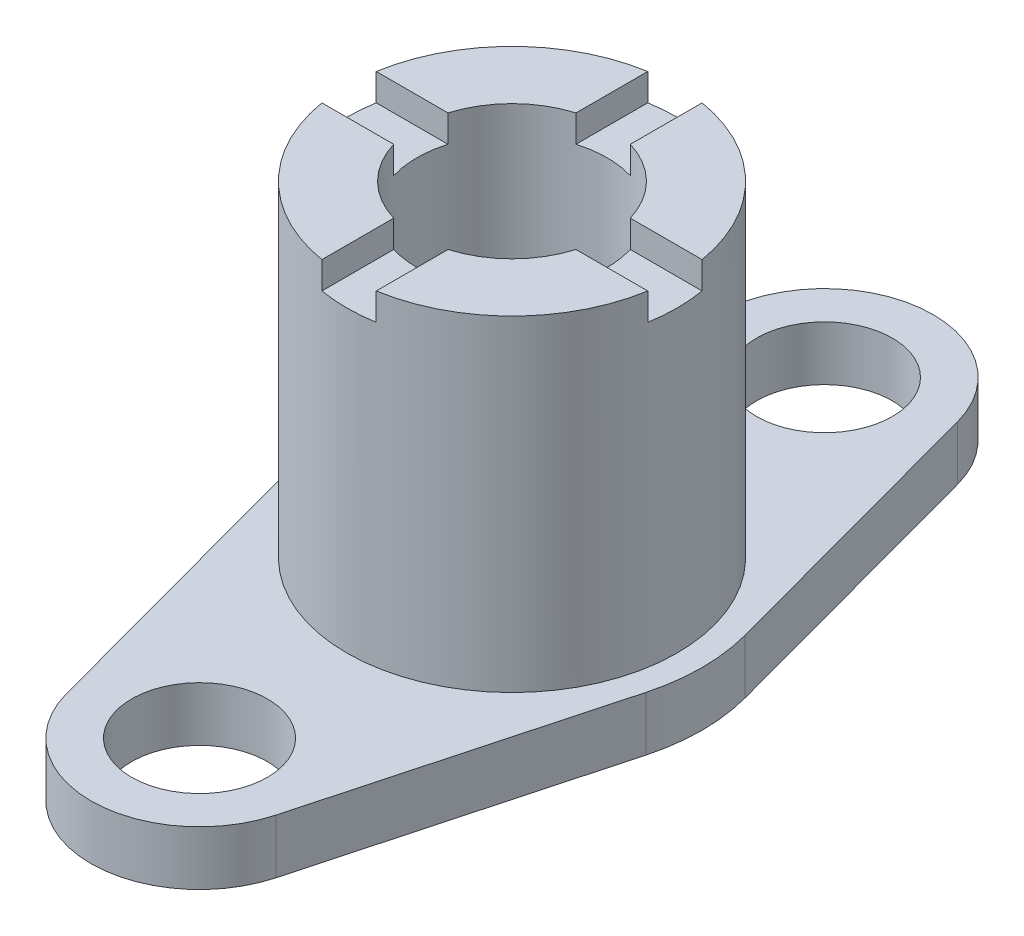
ISO-10303-21;
HEADER;
FILE_DESCRIPTION(('STEP AP214'),'2;1');
FILE_NAME('part.step','',(''),(''),'','','');
FILE_SCHEMA(('AUTOMOTIVE_DESIGN { 1 0 10303 214 1 1 1 1 }'));
ENDSEC;
DATA;
#1=APPLICATION_CONTEXT('core data for automotive mechanical design processes');
#2=APPLICATION_PROTOCOL_DEFINITION('international standard','automotive_design',2000,#1);
#3=PRODUCT_CONTEXT('',#1,'mechanical');
#4=PRODUCT('Part','Part','',(#3));
#5=PRODUCT_RELATED_PRODUCT_CATEGORY('part','',(#4));
#6=PRODUCT_DEFINITION_FORMATION('','',#4);
#7=PRODUCT_DEFINITION_CONTEXT('part definition',#1,'design');
#8=PRODUCT_DEFINITION('design','',#6,#7);
#9=PRODUCT_DEFINITION_SHAPE('','',#8);
#10=(LENGTH_UNIT() NAMED_UNIT(*) SI_UNIT(.MILLI.,.METRE.));
#11=(NAMED_UNIT(*) PLANE_ANGLE_UNIT() SI_UNIT($,.RADIAN.));
#12=(NAMED_UNIT(*) SI_UNIT($,.STERADIAN.) SOLID_ANGLE_UNIT());
#13=UNCERTAINTY_MEASURE_WITH_UNIT(LENGTH_MEASURE(1.E-05),#10,'distance_accuracy_value','');
#14=(GEOMETRIC_REPRESENTATION_CONTEXT(3) GLOBAL_UNCERTAINTY_ASSIGNED_CONTEXT((#13)) GLOBAL_UNIT_ASSIGNED_CONTEXT((#10,
#11,#12)) REPRESENTATION_CONTEXT('',''));
#15=CARTESIAN_POINT('',(0.,0.,0.));
#16=DIRECTION('',(0.,0.,1.));
#17=DIRECTION('',(1.,0.,0.));
#18=AXIS2_PLACEMENT_3D('',#15,#16,#17);
#19=CARTESIAN_POINT('',(0.,70.,0.));
#20=DIRECTION('',(0.,1.,0.));
#21=DIRECTION('',(0.,0.,1.));
#22=AXIS2_PLACEMENT_3D('',#19,#20,#21);
#23=PLANE('',#22);
#24=DIRECTION('',(1.,0.,0.));
#25=VECTOR('',#24,1.);
#26=CARTESIAN_POINT('',(-16.7705098312484,70.,4.99999999999994));
#27=LINE('',#26,#25);
#28=CARTESIAN_POINT('',(-29.9810977207389,70.,4.9999999999999));
#29=VERTEX_POINT('',#28);
#30=CARTESIAN_POINT('',(-16.7705098312484,70.,4.99999999999994));
#31=VERTEX_POINT('',#30);
#32=EDGE_CURVE('E216',#29,#31,#27,.T.);
#33=ORIENTED_EDGE('',*,*,#32,.F.);
#34=CARTESIAN_POINT('',(0.,70.,0.));
#35=DIRECTION('',(0.,1.,0.));
#36=DIRECTION('',(0.,0.,1.));
#37=AXIS2_PLACEMENT_3D('',#34,#35,#36);
#38=CIRCLE('',#37,30.3951677169331);
#39=CARTESIAN_POINT('',(-5.,70.,29.9810977207388));
#40=VERTEX_POINT('',#39);
#41=EDGE_CURVE('E311',#29,#40,#38,.T.);
#42=ORIENTED_EDGE('',*,*,#41,.T.);
#43=DIRECTION('',(0.,0.,1.));
#44=VECTOR('',#43,1.);
#45=CARTESIAN_POINT('',(-5.,70.,16.7705098312484));
#46=LINE('',#45,#44);
#47=CARTESIAN_POINT('',(-5.,70.,16.7705098312484));
#48=VERTEX_POINT('',#47);
#49=EDGE_CURVE('E244',#48,#40,#46,.T.);
#50=ORIENTED_EDGE('',*,*,#49,.F.);
#51=CARTESIAN_POINT('',(0.,70.,0.));
#52=DIRECTION('',(0.,1.,0.));
#53=DIRECTION('',(0.,0.,1.));
#54=AXIS2_PLACEMENT_3D('',#51,#52,#53);
#55=CIRCLE('',#54,17.5);
#56=EDGE_CURVE('E305',#31,#48,#55,.T.);
#57=ORIENTED_EDGE('',*,*,#56,.F.);
#58=EDGE_LOOP('',(#33,#42,#50,#57));
#59=FACE_BOUND('',#58,.T.);
#60=ADVANCED_FACE('F39',(#59),#23,.T.);
#61=DIRECTION('',(0.,0.,-1.));
#62=VECTOR('',#61,1.);
#63=CARTESIAN_POINT('',(5.,70.,16.7705098312484));
#64=LINE('',#63,#62);
#65=CARTESIAN_POINT('',(5.,70.,29.9810977207388));
#66=VERTEX_POINT('',#65);
#67=CARTESIAN_POINT('',(5.,70.,16.7705098312484));
#68=VERTEX_POINT('',#67);
#69=EDGE_CURVE('E238',#66,#68,#64,.T.);
#70=ORIENTED_EDGE('',*,*,#69,.F.);
#71=CARTESIAN_POINT('',(29.9810977207388,70.,5.00000000000032));
#72=VERTEX_POINT('',#71);
#73=EDGE_CURVE('E306',#66,#72,#38,.T.);
#74=ORIENTED_EDGE('',*,*,#73,.T.);
#75=DIRECTION('',(1.,0.,0.));
#76=VECTOR('',#75,1.);
#77=CARTESIAN_POINT('',(16.7705098312484,70.,5.00000000000018));
#78=LINE('',#77,#76);
#79=CARTESIAN_POINT('',(16.7705098312484,70.,5.00000000000018));
#80=VERTEX_POINT('',#79);
#81=EDGE_CURVE('E263',#80,#72,#78,.T.);
#82=ORIENTED_EDGE('',*,*,#81,.F.);
#83=EDGE_CURVE('E296',#68,#80,#55,.T.);
#84=ORIENTED_EDGE('',*,*,#83,.F.);
#85=EDGE_LOOP('',(#70,#74,#82,#84));
#86=FACE_BOUND('',#85,.T.);
#87=ADVANCED_FACE('F427',(#86),#23,.T.);
#88=DIRECTION('',(-1.,0.,0.));
#89=VECTOR('',#88,1.);
#90=CARTESIAN_POINT('',(-16.7705098312484,70.,-5.00000000000006));
#91=LINE('',#90,#89);
#92=CARTESIAN_POINT('',(-16.7705098312484,70.,-5.00000000000006));
#93=VERTEX_POINT('',#92);
#94=CARTESIAN_POINT('',(-29.9810977207388,70.,-5.00000000000011));
#95=VERTEX_POINT('',#94);
#96=EDGE_CURVE('E243',#93,#95,#91,.T.);
#97=ORIENTED_EDGE('',*,*,#96,.F.);
#98=CARTESIAN_POINT('',(-4.99999999999988,70.,-16.7705098312485));
#99=VERTEX_POINT('',#98);
#100=EDGE_CURVE('E225',#99,#93,#55,.T.);
#101=ORIENTED_EDGE('',*,*,#100,.F.);
#102=DIRECTION('',(0.,0.,1.));
#103=VECTOR('',#102,1.);
#104=CARTESIAN_POINT('',(-4.99999999999988,70.,-16.7705098312485));
#105=LINE('',#104,#103);
#106=CARTESIAN_POINT('',(-4.99999999999979,70.,-29.9810977207389));
#107=VERTEX_POINT('',#106);
#108=EDGE_CURVE('E262',#107,#99,#105,.T.);
#109=ORIENTED_EDGE('',*,*,#108,.F.);
#110=EDGE_CURVE('E464',#107,#95,#38,.T.);
#111=ORIENTED_EDGE('',*,*,#110,.T.);
#112=EDGE_LOOP('',(#97,#101,#109,#111));
#113=FACE_BOUND('',#112,.T.);
#114=ADVANCED_FACE('F440',(#113),#23,.T.);
#115=CARTESIAN_POINT('',(0.,10.,57.5));
#116=DIRECTION('',(0.,-1.,0.));
#117=DIRECTION('',(0.,0.,-1.));
#118=AXIS2_PLACEMENT_3D('',#115,#116,#117);
#119=CYLINDRICAL_SURFACE('',#118,20.);
#120=CARTESIAN_POINT('',(0.,0.,57.5));
#121=DIRECTION('',(0.,1.,0.));
#122=DIRECTION('',(0.,0.,1.));
#123=AXIS2_PLACEMENT_3D('',#120,#121,#122);
#124=CIRCLE('',#123,20.);
#125=CARTESIAN_POINT('',(-19.3074811401518,0.,62.7173913043478));
#126=VERTEX_POINT('',#125);
#127=CARTESIAN_POINT('',(19.3074811401518,0.,62.7173913043478));
#128=VERTEX_POINT('',#127);
#129=EDGE_CURVE('E317',#126,#128,#124,.T.);
#130=ORIENTED_EDGE('',*,*,#129,.T.);
#131=DIRECTION('',(0.,-1.,0.));
#132=VECTOR('',#131,1.);
#133=CARTESIAN_POINT('',(19.3074811401518,10.,62.7173913043478));
#134=LINE('',#133,#132);
#135=CARTESIAN_POINT('',(19.3074811401518,10.,62.7173913043478));
#136=VERTEX_POINT('',#135);
#137=EDGE_CURVE('E11',#136,#128,#134,.T.);
#138=ORIENTED_EDGE('',*,*,#137,.F.);
#139=CARTESIAN_POINT('',(0.,10.,57.5));
#140=DIRECTION('',(0.,1.,0.));
#141=DIRECTION('',(0.,0.,1.));
#142=AXIS2_PLACEMENT_3D('',#139,#140,#141);
#143=CIRCLE('',#142,20.);
#144=CARTESIAN_POINT('',(-19.3074811401518,10.,62.7173913043478));
#145=VERTEX_POINT('',#144);
#146=EDGE_CURVE('E327',#145,#136,#143,.T.);
#147=ORIENTED_EDGE('',*,*,#146,.F.);
#148=DIRECTION('',(0.,-1.,0.));
#149=VECTOR('',#148,1.);
#150=CARTESIAN_POINT('',(-19.3074811401518,10.,62.7173913043478));
#151=LINE('',#150,#149);
#152=EDGE_CURVE('E347',#145,#126,#151,.T.);
#153=ORIENTED_EDGE('',*,*,#152,.T.);
#154=EDGE_LOOP('',(#130,#138,#147,#153));
#155=FACE_BOUND('',#154,.T.);
#156=ADVANCED_FACE('F41',(#155),#119,.T.);
#157=CARTESIAN_POINT('',(19.3074811401518,10.,62.7173913043478));
#158=DIRECTION('',(-0.965374057007588,0.,-0.260869565217391));
#159=DIRECTION('',(-0.260869565217391,0.,0.965374057007588));
#160=AXIS2_PLACEMENT_3D('',#157,#158,#159);
#161=PLANE('',#160);
#162=DIRECTION('',(0.260869565217391,0.,-0.965374057007588));
#163=VECTOR('',#162,1.);
#164=CARTESIAN_POINT('',(19.3074811401518,0.,62.7173913043478));
#165=LINE('',#164,#163);
#166=CARTESIAN_POINT('',(33.7880919952656,0.,9.13043478260872));
#167=VERTEX_POINT('',#166);
#168=EDGE_CURVE('E349',#128,#167,#165,.T.);
#169=ORIENTED_EDGE('',*,*,#168,.T.);
#170=DIRECTION('',(0.,-1.,0.));
#171=VECTOR('',#170,1.);
#172=CARTESIAN_POINT('',(33.7880919952656,10.,9.13043478260872));
#173=LINE('',#172,#171);
#174=CARTESIAN_POINT('',(33.7880919952656,10.,9.13043478260872));
#175=VERTEX_POINT('',#174);
#176=EDGE_CURVE('E50',#175,#167,#173,.T.);
#177=ORIENTED_EDGE('',*,*,#176,.F.);
#178=DIRECTION('',(0.260869565217391,0.,-0.965374057007588));
#179=VECTOR('',#178,1.);
#180=CARTESIAN_POINT('',(19.3074811401518,10.,62.7173913043478));
#181=LINE('',#180,#179);
#182=EDGE_CURVE('E332',#136,#175,#181,.T.);
#183=ORIENTED_EDGE('',*,*,#182,.F.);
#184=ORIENTED_EDGE('',*,*,#137,.T.);
#185=EDGE_LOOP('',(#169,#177,#183,#184));
#186=FACE_BOUND('',#185,.T.);
#187=ADVANCED_FACE('F407',(#186),#161,.F.);
#188=CARTESIAN_POINT('',(0.,10.,0.));
#189=DIRECTION('',(0.,-1.,0.));
#190=DIRECTION('',(0.,0.,-1.));
#191=AXIS2_PLACEMENT_3D('',#188,#189,#190);
#192=CYLINDRICAL_SURFACE('',#191,35.);
#193=CARTESIAN_POINT('',(0.,0.,0.));
#194=DIRECTION('',(0.,1.,0.));
#195=DIRECTION('',(0.,0.,1.));
#196=AXIS2_PLACEMENT_3D('',#193,#194,#195);
#197=CIRCLE('',#196,35.);
#198=CARTESIAN_POINT('',(33.7880919952656,0.,-9.13043478260871));
#199=VERTEX_POINT('',#198);
#200=EDGE_CURVE('E352',#167,#199,#197,.T.);
#201=ORIENTED_EDGE('',*,*,#200,.T.);
#202=DIRECTION('',(0.,-1.,0.));
#203=VECTOR('',#202,1.);
#204=CARTESIAN_POINT('',(33.7880919952656,10.,-9.13043478260871));
#205=LINE('',#204,#203);
#206=CARTESIAN_POINT('',(33.7880919952656,10.,-9.13043478260871));
#207=VERTEX_POINT('',#206);
#208=EDGE_CURVE('E376',#207,#199,#205,.T.);
#209=ORIENTED_EDGE('',*,*,#208,.F.);
#210=CARTESIAN_POINT('',(0.,10.,0.));
#211=DIRECTION('',(0.,1.,0.));
#212=DIRECTION('',(0.,0.,1.));
#213=AXIS2_PLACEMENT_3D('',#210,#211,#212);
#214=CIRCLE('',#213,35.);
#215=EDGE_CURVE('E331',#175,#207,#214,.T.);
#216=ORIENTED_EDGE('',*,*,#215,.F.);
#217=ORIENTED_EDGE('',*,*,#176,.T.);
#218=EDGE_LOOP('',(#201,#209,#216,#217));
#219=FACE_BOUND('',#218,.T.);
#220=ADVANCED_FACE('F382',(#219),#192,.T.);
#221=CARTESIAN_POINT('',(19.3074811401517,10.,-62.7173913043478));
#222=DIRECTION('',(-0.965374057007588,0.,0.260869565217392));
#223=DIRECTION('',(0.260869565217392,0.,0.965374057007588));
#224=AXIS2_PLACEMENT_3D('',#221,#222,#223);
#225=PLANE('',#224);
#226=DIRECTION('',(-0.260869565217392,0.,-0.965374057007588));
#227=VECTOR('',#226,1.);
#228=CARTESIAN_POINT('',(19.3074811401517,0.,-62.7173913043478));
#229=LINE('',#228,#227);
#230=CARTESIAN_POINT('',(19.3074811401517,0.,-62.7173913043478));
#231=VERTEX_POINT('',#230);
#232=EDGE_CURVE('E355',#199,#231,#229,.T.);
#233=ORIENTED_EDGE('',*,*,#232,.T.);
#234=DIRECTION('',(0.,-1.,0.));
#235=VECTOR('',#234,1.);
#236=CARTESIAN_POINT('',(19.3074811401517,10.,-62.7173913043478));
#237=LINE('',#236,#235);
#238=CARTESIAN_POINT('',(19.3074811401517,10.,-62.7173913043478));
#239=VERTEX_POINT('',#238);
#240=EDGE_CURVE('E373',#239,#231,#237,.T.);
#241=ORIENTED_EDGE('',*,*,#240,.F.);
#242=DIRECTION('',(-0.260869565217392,0.,-0.965374057007588));
#243=VECTOR('',#242,1.);
#244=CARTESIAN_POINT('',(19.3074811401517,10.,-62.7173913043478));
#245=LINE('',#244,#243);
#246=EDGE_CURVE('E337',#207,#239,#245,.T.);
#247=ORIENTED_EDGE('',*,*,#246,.F.);
#248=ORIENTED_EDGE('',*,*,#208,.T.);
#249=EDGE_LOOP('',(#233,#241,#247,#248));
#250=FACE_BOUND('',#249,.T.);
#251=ADVANCED_FACE('F391',(#250),#225,.F.);
#252=CARTESIAN_POINT('',(0.,10.,-57.5));
#253=DIRECTION('',(0.,-1.,0.));
#254=DIRECTION('',(0.,0.,-1.));
#255=AXIS2_PLACEMENT_3D('',#252,#253,#254);
#256=CYLINDRICAL_SURFACE('',#255,20.);
#257=CARTESIAN_POINT('',(0.,0.,-57.5));
#258=DIRECTION('',(0.,1.,0.));
#259=DIRECTION('',(0.,0.,1.));
#260=AXIS2_PLACEMENT_3D('',#257,#258,#259);
#261=CIRCLE('',#260,20.);
#262=CARTESIAN_POINT('',(-19.3074811401518,0.,-62.7173913043478));
#263=VERTEX_POINT('',#262);
#264=EDGE_CURVE('E353',#231,#263,#261,.T.);
#265=ORIENTED_EDGE('',*,*,#264,.T.);
#266=DIRECTION('',(0.,-1.,0.));
#267=VECTOR('',#266,1.);
#268=CARTESIAN_POINT('',(-19.3074811401518,10.,-62.7173913043478));
#269=LINE('',#268,#267);
#270=CARTESIAN_POINT('',(-19.3074811401518,10.,-62.7173913043478));
#271=VERTEX_POINT('',#270);
#272=EDGE_CURVE('E367',#271,#263,#269,.T.);
#273=ORIENTED_EDGE('',*,*,#272,.F.);
#274=CARTESIAN_POINT('',(0.,10.,-57.5));
#275=DIRECTION('',(0.,1.,0.));
#276=DIRECTION('',(0.,0.,1.));
#277=AXIS2_PLACEMENT_3D('',#274,#275,#276);
#278=CIRCLE('',#277,20.);
#279=EDGE_CURVE('E340',#239,#271,#278,.T.);
#280=ORIENTED_EDGE('',*,*,#279,.F.);
#281=ORIENTED_EDGE('',*,*,#240,.T.);
#282=EDGE_LOOP('',(#265,#273,#280,#281));
#283=FACE_BOUND('',#282,.T.);
#284=ADVANCED_FACE('F397',(#283),#256,.T.);
#285=CARTESIAN_POINT('',(-19.3074811401518,10.,-62.7173913043478));
#286=DIRECTION('',(0.965374057007588,0.,0.260869565217391));
#287=DIRECTION('',(0.260869565217391,0.,-0.965374057007588));
#288=AXIS2_PLACEMENT_3D('',#285,#286,#287);
#289=PLANE('',#288);
#290=DIRECTION('',(-0.260869565217391,0.,0.965374057007588));
#291=VECTOR('',#290,1.);
#292=CARTESIAN_POINT('',(-19.3074811401518,0.,-62.7173913043478));
#293=LINE('',#292,#291);
#294=CARTESIAN_POINT('',(-33.7880919952656,0.,-9.13043478260871));
#295=VERTEX_POINT('',#294);
#296=EDGE_CURVE('E359',#263,#295,#293,.T.);
#297=ORIENTED_EDGE('',*,*,#296,.T.);
#298=DIRECTION('',(0.,-1.,0.));
#299=VECTOR('',#298,1.);
#300=CARTESIAN_POINT('',(-33.7880919952656,10.,-9.13043478260871));
#301=LINE('',#300,#299);
#302=CARTESIAN_POINT('',(-33.7880919952656,10.,-9.13043478260871));
#303=VERTEX_POINT('',#302);
#304=EDGE_CURVE('E370',#303,#295,#301,.T.);
#305=ORIENTED_EDGE('',*,*,#304,.F.);
#306=DIRECTION('',(-0.260869565217391,0.,0.965374057007588));
#307=VECTOR('',#306,1.);
#308=CARTESIAN_POINT('',(-19.3074811401518,10.,-62.7173913043478));
#309=LINE('',#308,#307);
#310=EDGE_CURVE('E338',#271,#303,#309,.T.);
#311=ORIENTED_EDGE('',*,*,#310,.F.);
#312=ORIENTED_EDGE('',*,*,#272,.T.);
#313=EDGE_LOOP('',(#297,#305,#311,#312));
#314=FACE_BOUND('',#313,.T.);
#315=ADVANCED_FACE('F420',(#314),#289,.F.);
#316=CARTESIAN_POINT('',(0.,10.,0.));
#317=DIRECTION('',(0.,-1.,0.));
#318=DIRECTION('',(0.,0.,-1.));
#319=AXIS2_PLACEMENT_3D('',#316,#317,#318);
#320=CYLINDRICAL_SURFACE('',#319,35.);
#321=CARTESIAN_POINT('',(0.,0.,0.));
#322=DIRECTION('',(0.,1.,0.));
#323=DIRECTION('',(0.,0.,1.));
#324=AXIS2_PLACEMENT_3D('',#321,#322,#323);
#325=CIRCLE('',#324,35.);
#326=CARTESIAN_POINT('',(-33.7880919952656,0.,9.13043478260873));
#327=VERTEX_POINT('',#326);
#328=EDGE_CURVE('E360',#295,#327,#325,.T.);
#329=ORIENTED_EDGE('',*,*,#328,.T.);
#330=DIRECTION('',(0.,-1.,0.));
#331=VECTOR('',#330,1.);
#332=CARTESIAN_POINT('',(-33.7880919952656,10.,9.13043478260873));
#333=LINE('',#332,#331);
#334=CARTESIAN_POINT('',(-33.7880919952656,10.,9.13043478260873));
#335=VERTEX_POINT('',#334);
#336=EDGE_CURVE('E365',#335,#327,#333,.T.);
#337=ORIENTED_EDGE('',*,*,#336,.F.);
#338=CARTESIAN_POINT('',(0.,10.,0.));
#339=DIRECTION('',(0.,1.,0.));
#340=DIRECTION('',(0.,0.,1.));
#341=AXIS2_PLACEMENT_3D('',#338,#339,#340);
#342=CIRCLE('',#341,35.);
#343=EDGE_CURVE('E344',#303,#335,#342,.T.);
#344=ORIENTED_EDGE('',*,*,#343,.F.);
#345=ORIENTED_EDGE('',*,*,#304,.T.);
#346=EDGE_LOOP('',(#329,#337,#344,#345));
#347=FACE_BOUND('',#346,.T.);
#348=ADVANCED_FACE('F417',(#347),#320,.T.);
#349=CARTESIAN_POINT('',(-19.3074811401518,10.,62.7173913043478));
#350=DIRECTION('',(0.965374057007588,0.,-0.260869565217391));
#351=DIRECTION('',(-0.260869565217391,0.,-0.965374057007588));
#352=AXIS2_PLACEMENT_3D('',#349,#350,#351);
#353=PLANE('',#352);
#354=DIRECTION('',(0.260869565217391,0.,0.965374057007588));
#355=VECTOR('',#354,1.);
#356=CARTESIAN_POINT('',(-19.3074811401518,0.,62.7173913043478));
#357=LINE('',#356,#355);
#358=EDGE_CURVE('E335',#327,#126,#357,.T.);
#359=ORIENTED_EDGE('',*,*,#358,.T.);
#360=ORIENTED_EDGE('',*,*,#152,.F.);
#361=DIRECTION('',(0.260869565217391,0.,0.965374057007588));
#362=VECTOR('',#361,1.);
#363=CARTESIAN_POINT('',(-19.3074811401518,10.,62.7173913043478));
#364=LINE('',#363,#362);
#365=EDGE_CURVE('E345',#335,#145,#364,.T.);
#366=ORIENTED_EDGE('',*,*,#365,.F.);
#367=ORIENTED_EDGE('',*,*,#336,.T.);
#368=EDGE_LOOP('',(#359,#360,#366,#367));
#369=FACE_BOUND('',#368,.T.);
#370=ADVANCED_FACE('F414',(#369),#353,.F.);
#371=CARTESIAN_POINT('',(0.,10.,57.5));
#372=DIRECTION('',(0.,1.,0.));
#373=DIRECTION('',(0.,0.,1.));
#374=AXIS2_PLACEMENT_3D('',#371,#372,#373);
#375=PLANE('',#374);
#376=CARTESIAN_POINT('',(0.,10.,0.));
#377=DIRECTION('',(0.,1.,0.));
#378=DIRECTION('',(0.,0.,1.));
#379=AXIS2_PLACEMENT_3D('',#376,#377,#378);
#380=CIRCLE('',#379,30.3951677169331);
#381=CARTESIAN_POINT('',(0.,10.,30.3951677169331));
#382=VERTEX_POINT('',#381);
#383=EDGE_CURVE('E307',#382,#382,#380,.T.);
#384=ORIENTED_EDGE('',*,*,#383,.F.);
#385=EDGE_LOOP('',(#384));
#386=FACE_BOUND('',#385,.T.);
#387=CARTESIAN_POINT('',(0.,10.,-57.5));
#388=DIRECTION('',(0.,1.,0.));
#389=DIRECTION('',(0.,0.,1.));
#390=AXIS2_PLACEMENT_3D('',#387,#388,#389);
#391=CIRCLE('',#390,12.5);
#392=CARTESIAN_POINT('',(0.,10.,-45.));
#393=VERTEX_POINT('',#392);
#394=EDGE_CURVE('E319',#393,#393,#391,.T.);
#395=ORIENTED_EDGE('',*,*,#394,.F.);
#396=EDGE_LOOP('',(#395));
#397=FACE_BOUND('',#396,.T.);
#398=CARTESIAN_POINT('',(0.,10.,57.5));
#399=DIRECTION('',(0.,1.,0.));
#400=DIRECTION('',(0.,0.,1.));
#401=AXIS2_PLACEMENT_3D('',#398,#399,#400);
#402=CIRCLE('',#401,12.5);
#403=CARTESIAN_POINT('',(0.,10.,70.));
#404=VERTEX_POINT('',#403);
#405=EDGE_CURVE('E323',#404,#404,#402,.T.);
#406=ORIENTED_EDGE('',*,*,#405,.F.);
#407=EDGE_LOOP('',(#406));
#408=FACE_BOUND('',#407,.T.);
#409=ORIENTED_EDGE('',*,*,#146,.T.);
#410=ORIENTED_EDGE('',*,*,#182,.T.);
#411=ORIENTED_EDGE('',*,*,#215,.T.);
#412=ORIENTED_EDGE('',*,*,#246,.T.);
#413=ORIENTED_EDGE('',*,*,#279,.T.);
#414=ORIENTED_EDGE('',*,*,#310,.T.);
#415=ORIENTED_EDGE('',*,*,#343,.T.);
#416=ORIENTED_EDGE('',*,*,#365,.T.);
#417=EDGE_LOOP('',(#409,#410,#411,#412,#413,#414,#415,#416));
#418=FACE_BOUND('',#417,.T.);
#419=ADVANCED_FACE('F405',(#386,#397,#408,#418),#375,.T.);
#420=CARTESIAN_POINT('',(0.,0.,57.5));
#421=DIRECTION('',(0.,1.,0.));
#422=DIRECTION('',(0.,0.,1.));
#423=AXIS2_PLACEMENT_3D('',#420,#421,#422);
#424=PLANE('',#423);
#425=CARTESIAN_POINT('',(0.,0.,-57.5));
#426=DIRECTION('',(0.,1.,0.));
#427=DIRECTION('',(0.,0.,1.));
#428=AXIS2_PLACEMENT_3D('',#425,#426,#427);
#429=CIRCLE('',#428,12.5);
#430=CARTESIAN_POINT('',(0.,0.,-45.));
#431=VERTEX_POINT('',#430);
#432=EDGE_CURVE('E316',#431,#431,#429,.T.);
#433=ORIENTED_EDGE('',*,*,#432,.T.);
#434=EDGE_LOOP('',(#433));
#435=FACE_BOUND('',#434,.T.);
#436=CARTESIAN_POINT('',(0.,0.,57.5));
#437=DIRECTION('',(0.,1.,0.));
#438=DIRECTION('',(0.,0.,1.));
#439=AXIS2_PLACEMENT_3D('',#436,#437,#438);
#440=CIRCLE('',#439,12.5);
#441=CARTESIAN_POINT('',(0.,0.,70.));
#442=VERTEX_POINT('',#441);
#443=EDGE_CURVE('E313',#442,#442,#440,.T.);
#444=ORIENTED_EDGE('',*,*,#443,.T.);
#445=EDGE_LOOP('',(#444));
#446=FACE_BOUND('',#445,.T.);
#447=ORIENTED_EDGE('',*,*,#129,.F.);
#448=ORIENTED_EDGE('',*,*,#358,.F.);
#449=ORIENTED_EDGE('',*,*,#328,.F.);
#450=ORIENTED_EDGE('',*,*,#296,.F.);
#451=ORIENTED_EDGE('',*,*,#264,.F.);
#452=ORIENTED_EDGE('',*,*,#232,.F.);
#453=ORIENTED_EDGE('',*,*,#200,.F.);
#454=ORIENTED_EDGE('',*,*,#168,.F.);
#455=EDGE_LOOP('',(#447,#448,#449,#450,#451,#452,#453,#454));
#456=FACE_BOUND('',#455,.T.);
#457=ADVANCED_FACE('F386',(#435,#446,#456),#424,.F.);
#458=CARTESIAN_POINT('',(0.,0.,57.5));
#459=DIRECTION('',(0.,1.,0.));
#460=DIRECTION('',(0.,0.,1.));
#461=AXIS2_PLACEMENT_3D('',#458,#459,#460);
#462=CYLINDRICAL_SURFACE('',#461,12.5);
#463=ORIENTED_EDGE('',*,*,#443,.F.);
#464=EDGE_LOOP('',(#463));
#465=FACE_BOUND('',#464,.T.);
#466=ORIENTED_EDGE('',*,*,#405,.T.);
#467=EDGE_LOOP('',(#466));
#468=FACE_BOUND('',#467,.T.);
#469=ADVANCED_FACE('F557',(#465,#468),#462,.F.);
#470=CARTESIAN_POINT('',(0.,0.,-57.5));
#471=DIRECTION('',(0.,1.,0.));
#472=DIRECTION('',(0.,0.,1.));
#473=AXIS2_PLACEMENT_3D('',#470,#471,#472);
#474=CYLINDRICAL_SURFACE('',#473,12.5);
#475=ORIENTED_EDGE('',*,*,#432,.F.);
#476=EDGE_LOOP('',(#475));
#477=FACE_BOUND('',#476,.T.);
#478=ORIENTED_EDGE('',*,*,#394,.T.);
#479=EDGE_LOOP('',(#478));
#480=FACE_BOUND('',#479,.T.);
#481=ADVANCED_FACE('F453',(#477,#480),#474,.F.);
#482=CARTESIAN_POINT('',(0.,70.,0.));
#483=DIRECTION('',(0.,-1.,0.));
#484=DIRECTION('',(0.,0.,-1.));
#485=AXIS2_PLACEMENT_3D('',#482,#483,#484);
#486=CYLINDRICAL_SURFACE('',#485,30.3951677169331);
#487=ORIENTED_EDGE('',*,*,#41,.F.);
#488=DIRECTION('',(0.,1.,0.));
#489=VECTOR('',#488,1.);
#490=CARTESIAN_POINT('',(-29.9810977207389,65.,4.9999999999999));
#491=LINE('',#490,#489);
#492=CARTESIAN_POINT('',(-29.9810977207389,65.,4.9999999999999));
#493=VERTEX_POINT('',#492);
#494=EDGE_CURVE('E221',#493,#29,#491,.T.);
#495=ORIENTED_EDGE('',*,*,#494,.F.);
#496=CARTESIAN_POINT('',(0.,65.,0.));
#497=DIRECTION('',(0.,1.,0.));
#498=DIRECTION('',(0.,0.,1.));
#499=AXIS2_PLACEMENT_3D('',#496,#497,#498);
#500=CIRCLE('',#499,30.3951677169331);
#501=CARTESIAN_POINT('',(-29.9810977207388,65.,-5.00000000000011));
#502=VERTEX_POINT('',#501);
#503=EDGE_CURVE('E207',#502,#493,#500,.T.);
#504=ORIENTED_EDGE('',*,*,#503,.F.);
#505=DIRECTION('',(0.,1.,0.));
#506=VECTOR('',#505,1.);
#507=CARTESIAN_POINT('',(-29.9810977207388,65.,-5.00000000000011));
#508=LINE('',#507,#506);
#509=EDGE_CURVE('E210',#502,#95,#508,.T.);
#510=ORIENTED_EDGE('',*,*,#509,.T.);
#511=ORIENTED_EDGE('',*,*,#110,.F.);
#512=DIRECTION('',(0.,1.,0.));
#513=VECTOR('',#512,1.);
#514=CARTESIAN_POINT('',(-4.99999999999979,65.,-29.9810977207389));
#515=LINE('',#514,#513);
#516=CARTESIAN_POINT('',(-4.99999999999979,65.,-29.9810977207389));
#517=VERTEX_POINT('',#516);
#518=EDGE_CURVE('E259',#517,#107,#515,.T.);
#519=ORIENTED_EDGE('',*,*,#518,.F.);
#520=CARTESIAN_POINT('',(0.,65.,0.));
#521=DIRECTION('',(0.,1.,0.));
#522=DIRECTION('',(0.,0.,1.));
#523=AXIS2_PLACEMENT_3D('',#520,#521,#522);
#524=CIRCLE('',#523,30.3951677169331);
#525=CARTESIAN_POINT('',(5.00000000000021,65.,-29.9810977207388));
#526=VERTEX_POINT('',#525);
#527=EDGE_CURVE('E267',#526,#517,#524,.T.);
#528=ORIENTED_EDGE('',*,*,#527,.F.);
#529=DIRECTION('',(0.,1.,0.));
#530=VECTOR('',#529,1.);
#531=CARTESIAN_POINT('',(5.00000000000021,65.,-29.9810977207388));
#532=LINE('',#531,#530);
#533=CARTESIAN_POINT('',(5.00000000000021,70.,-29.9810977207388));
#534=VERTEX_POINT('',#533);
#535=EDGE_CURVE('E258',#526,#534,#532,.T.);
#536=ORIENTED_EDGE('',*,*,#535,.T.);
#537=CARTESIAN_POINT('',(29.9810977207389,70.,-4.99999999999968));
#538=VERTEX_POINT('',#537);
#539=EDGE_CURVE('E315',#538,#534,#38,.T.);
#540=ORIENTED_EDGE('',*,*,#539,.F.);
#541=DIRECTION('',(0.,1.,0.));
#542=VECTOR('',#541,1.);
#543=CARTESIAN_POINT('',(29.9810977207389,65.,-4.99999999999968));
#544=LINE('',#543,#542);
#545=CARTESIAN_POINT('',(29.9810977207389,65.,-4.99999999999968));
#546=VERTEX_POINT('',#545);
#547=EDGE_CURVE('E284',#546,#538,#544,.T.);
#548=ORIENTED_EDGE('',*,*,#547,.F.);
#549=CARTESIAN_POINT('',(0.,65.,0.));
#550=DIRECTION('',(0.,1.,0.));
#551=DIRECTION('',(0.,0.,1.));
#552=AXIS2_PLACEMENT_3D('',#549,#550,#551);
#553=CIRCLE('',#552,30.3951677169331);
#554=CARTESIAN_POINT('',(29.9810977207388,65.,5.00000000000032));
#555=VERTEX_POINT('',#554);
#556=EDGE_CURVE('E295',#555,#546,#553,.T.);
#557=ORIENTED_EDGE('',*,*,#556,.F.);
#558=DIRECTION('',(0.,1.,0.));
#559=VECTOR('',#558,1.);
#560=CARTESIAN_POINT('',(29.9810977207388,65.,5.00000000000032));
#561=LINE('',#560,#559);
#562=EDGE_CURVE('E276',#555,#72,#561,.T.);
#563=ORIENTED_EDGE('',*,*,#562,.T.);
#564=ORIENTED_EDGE('',*,*,#73,.F.);
#565=DIRECTION('',(0.,1.,0.));
#566=VECTOR('',#565,1.);
#567=CARTESIAN_POINT('',(5.,65.,29.9810977207388));
#568=LINE('',#567,#566);
#569=CARTESIAN_POINT('',(5.,65.,29.9810977207388));
#570=VERTEX_POINT('',#569);
#571=EDGE_CURVE('E235',#570,#66,#568,.T.);
#572=ORIENTED_EDGE('',*,*,#571,.F.);
#573=CARTESIAN_POINT('',(0.,65.,0.));
#574=DIRECTION('',(0.,1.,0.));
#575=DIRECTION('',(0.,0.,1.));
#576=AXIS2_PLACEMENT_3D('',#573,#574,#575);
#577=CIRCLE('',#576,30.3951677169331);
#578=CARTESIAN_POINT('',(-5.,65.,29.9810977207388));
#579=VERTEX_POINT('',#578);
#580=EDGE_CURVE('E249',#579,#570,#577,.T.);
#581=ORIENTED_EDGE('',*,*,#580,.F.);
#582=DIRECTION('',(0.,1.,0.));
#583=VECTOR('',#582,1.);
#584=CARTESIAN_POINT('',(-5.,65.,29.9810977207388));
#585=LINE('',#584,#583);
#586=EDGE_CURVE('E233',#579,#40,#585,.T.);
#587=ORIENTED_EDGE('',*,*,#586,.T.);
#588=EDGE_LOOP('',(#487,#495,#504,#510,#511,#519,#528,#536,#540,#548,#557,#563,#564,#572,#581,#587));
#589=FACE_BOUND('',#588,.T.);
#590=ORIENTED_EDGE('',*,*,#383,.T.);
#591=EDGE_LOOP('',(#590));
#592=FACE_BOUND('',#591,.T.);
#593=ADVANCED_FACE('F444',(#589,#592),#486,.T.);
#594=DIRECTION('',(0.,0.,-1.));
#595=VECTOR('',#594,1.);
#596=CARTESIAN_POINT('',(5.00000000000012,70.,-16.7705098312484));
#597=LINE('',#596,#595);
#598=CARTESIAN_POINT('',(5.00000000000012,70.,-16.7705098312484));
#599=VERTEX_POINT('',#598);
#600=EDGE_CURVE('E239',#599,#534,#597,.T.);
#601=ORIENTED_EDGE('',*,*,#600,.F.);
#602=CARTESIAN_POINT('',(16.7705098312485,70.,-4.99999999999982));
#603=VERTEX_POINT('',#602);
#604=EDGE_CURVE('E302',#603,#599,#55,.T.);
#605=ORIENTED_EDGE('',*,*,#604,.F.);
#606=DIRECTION('',(-1.,0.,0.));
#607=VECTOR('',#606,1.);
#608=CARTESIAN_POINT('',(16.7705098312485,70.,-4.99999999999982));
#609=LINE('',#608,#607);
#610=EDGE_CURVE('E289',#538,#603,#609,.T.);
#611=ORIENTED_EDGE('',*,*,#610,.F.);
#612=ORIENTED_EDGE('',*,*,#539,.T.);
#613=EDGE_LOOP('',(#601,#605,#611,#612));
#614=FACE_BOUND('',#613,.T.);
#615=ADVANCED_FACE('F435',(#614),#23,.T.);
#616=CARTESIAN_POINT('',(0.,-39.4974746830583,0.));
#617=DIRECTION('',(0.,1.,0.));
#618=DIRECTION('',(0.,0.,1.));
#619=AXIS2_PLACEMENT_3D('',#616,#617,#618);
#620=CYLINDRICAL_SURFACE('',#619,17.5);
#621=CARTESIAN_POINT('',(0.,10.,0.));
#622=DIRECTION('',(0.,1.,0.));
#623=DIRECTION('',(0.,0.,1.));
#624=AXIS2_PLACEMENT_3D('',#621,#622,#623);
#625=CIRCLE('',#624,17.5);
#626=CARTESIAN_POINT('',(0.,10.,17.5));
#627=VERTEX_POINT('',#626);
#628=EDGE_CURVE('E304',#627,#627,#625,.F.);
#629=ORIENTED_EDGE('',*,*,#628,.T.);
#630=EDGE_LOOP('',(#629));
#631=FACE_BOUND('',#630,.T.);
#632=CARTESIAN_POINT('',(0.,65.,0.));
#633=DIRECTION('',(0.,-1.,0.));
#634=DIRECTION('',(0.,0.,1.));
#635=AXIS2_PLACEMENT_3D('',#632,#633,#634);
#636=CIRCLE('',#635,17.5);
#637=CARTESIAN_POINT('',(-16.7705098312484,65.,4.99999999999994));
#638=VERTEX_POINT('',#637);
#639=CARTESIAN_POINT('',(-16.7705098312484,65.,-5.00000000000006));
#640=VERTEX_POINT('',#639);
#641=EDGE_CURVE('E209',#638,#640,#636,.T.);
#642=ORIENTED_EDGE('',*,*,#641,.F.);
#643=DIRECTION('',(0.,1.,0.));
#644=VECTOR('',#643,1.);
#645=CARTESIAN_POINT('',(-16.7705098312484,65.,4.99999999999994));
#646=LINE('',#645,#644);
#647=EDGE_CURVE('E469',#638,#31,#646,.T.);
#648=ORIENTED_EDGE('',*,*,#647,.T.);
#649=ORIENTED_EDGE('',*,*,#56,.T.);
#650=DIRECTION('',(0.,1.,0.));
#651=VECTOR('',#650,1.);
#652=CARTESIAN_POINT('',(-5.,65.,16.7705098312484));
#653=LINE('',#652,#651);
#654=CARTESIAN_POINT('',(-5.,65.,16.7705098312484));
#655=VERTEX_POINT('',#654);
#656=EDGE_CURVE('E226',#655,#48,#653,.T.);
#657=ORIENTED_EDGE('',*,*,#656,.F.);
#658=CARTESIAN_POINT('',(0.,65.,0.));
#659=DIRECTION('',(0.,-1.,0.));
#660=DIRECTION('',(0.,0.,1.));
#661=AXIS2_PLACEMENT_3D('',#658,#659,#660);
#662=CIRCLE('',#661,17.5);
#663=CARTESIAN_POINT('',(5.,65.,16.7705098312484));
#664=VERTEX_POINT('',#663);
#665=EDGE_CURVE('E245',#664,#655,#662,.T.);
#666=ORIENTED_EDGE('',*,*,#665,.F.);
#667=DIRECTION('',(0.,1.,0.));
#668=VECTOR('',#667,1.);
#669=CARTESIAN_POINT('',(5.,65.,16.7705098312484));
#670=LINE('',#669,#668);
#671=EDGE_CURVE('E237',#664,#68,#670,.T.);
#672=ORIENTED_EDGE('',*,*,#671,.T.);
#673=ORIENTED_EDGE('',*,*,#83,.T.);
#674=DIRECTION('',(0.,1.,0.));
#675=VECTOR('',#674,1.);
#676=CARTESIAN_POINT('',(16.7705098312484,65.,5.00000000000018));
#677=LINE('',#676,#675);
#678=CARTESIAN_POINT('',(16.7705098312484,65.,5.00000000000018));
#679=VERTEX_POINT('',#678);
#680=EDGE_CURVE('E277',#679,#80,#677,.T.);
#681=ORIENTED_EDGE('',*,*,#680,.F.);
#682=CARTESIAN_POINT('',(0.,65.,0.));
#683=DIRECTION('',(0.,-1.,0.));
#684=DIRECTION('',(0.,0.,1.));
#685=AXIS2_PLACEMENT_3D('',#682,#683,#684);
#686=CIRCLE('',#685,17.5);
#687=CARTESIAN_POINT('',(16.7705098312485,65.,-4.99999999999982));
#688=VERTEX_POINT('',#687);
#689=EDGE_CURVE('E290',#688,#679,#686,.T.);
#690=ORIENTED_EDGE('',*,*,#689,.F.);
#691=DIRECTION('',(0.,1.,0.));
#692=VECTOR('',#691,1.);
#693=CARTESIAN_POINT('',(16.7705098312485,65.,-4.99999999999982));
#694=LINE('',#693,#692);
#695=EDGE_CURVE('E281',#688,#603,#694,.T.);
#696=ORIENTED_EDGE('',*,*,#695,.T.);
#697=ORIENTED_EDGE('',*,*,#604,.T.);
#698=DIRECTION('',(0.,1.,0.));
#699=VECTOR('',#698,1.);
#700=CARTESIAN_POINT('',(5.00000000000012,65.,-16.7705098312484));
#701=LINE('',#700,#699);
#702=CARTESIAN_POINT('',(5.00000000000012,65.,-16.7705098312484));
#703=VERTEX_POINT('',#702);
#704=EDGE_CURVE('E251',#703,#599,#701,.T.);
#705=ORIENTED_EDGE('',*,*,#704,.F.);
#706=CARTESIAN_POINT('',(0.,65.,0.));
#707=DIRECTION('',(0.,-1.,0.));
#708=DIRECTION('',(0.,0.,1.));
#709=AXIS2_PLACEMENT_3D('',#706,#707,#708);
#710=CIRCLE('',#709,17.5);
#711=CARTESIAN_POINT('',(-4.99999999999988,65.,-16.7705098312485));
#712=VERTEX_POINT('',#711);
#713=EDGE_CURVE('E266',#712,#703,#710,.T.);
#714=ORIENTED_EDGE('',*,*,#713,.F.);
#715=DIRECTION('',(0.,1.,0.));
#716=VECTOR('',#715,1.);
#717=CARTESIAN_POINT('',(-4.99999999999988,65.,-16.7705098312485));
#718=LINE('',#717,#716);
#719=EDGE_CURVE('E261',#712,#99,#718,.T.);
#720=ORIENTED_EDGE('',*,*,#719,.T.);
#721=ORIENTED_EDGE('',*,*,#100,.T.);
#722=DIRECTION('',(0.,1.,0.));
#723=VECTOR('',#722,1.);
#724=CARTESIAN_POINT('',(-16.7705098312484,65.,-5.00000000000006));
#725=LINE('',#724,#723);
#726=EDGE_CURVE('E204',#640,#93,#725,.T.);
#727=ORIENTED_EDGE('',*,*,#726,.F.);
#728=EDGE_LOOP('',(#642,#648,#649,#657,#666,#672,#673,#681,#690,#696,#697,#705,#714,#720,#721,#727));
#729=FACE_BOUND('',#728,.T.);
#730=ADVANCED_FACE('F218',(#631,#729),#620,.F.);
#731=CARTESIAN_POINT('',(0.,10.,57.5));
#732=DIRECTION('',(0.,1.,0.));
#733=DIRECTION('',(0.,0.,1.));
#734=AXIS2_PLACEMENT_3D('',#731,#732,#733);
#735=PLANE('',#734);
#736=ORIENTED_EDGE('',*,*,#628,.F.);
#737=EDGE_LOOP('',(#736));
#738=FACE_BOUND('',#737,.T.);
#739=ADVANCED_FACE('F446',(#738),#735,.T.);
#740=CARTESIAN_POINT('',(16.7705098312485,65.,-4.99999999999982));
#741=DIRECTION('',(0.,0.,-1.));
#742=DIRECTION('',(-1.,0.,0.));
#743=AXIS2_PLACEMENT_3D('',#740,#741,#742);
#744=PLANE('',#743);
#745=ORIENTED_EDGE('',*,*,#610,.T.);
#746=ORIENTED_EDGE('',*,*,#695,.F.);
#747=DIRECTION('',(-1.,0.,0.));
#748=VECTOR('',#747,1.);
#749=CARTESIAN_POINT('',(16.7705098312485,65.,-4.99999999999982));
#750=LINE('',#749,#748);
#751=EDGE_CURVE('E279',#546,#688,#750,.T.);
#752=ORIENTED_EDGE('',*,*,#751,.F.);
#753=ORIENTED_EDGE('',*,*,#547,.T.);
#754=EDGE_LOOP('',(#745,#746,#752,#753));
#755=FACE_BOUND('',#754,.T.);
#756=ADVANCED_FACE('F521',(#755),#744,.F.);
#757=CARTESIAN_POINT('',(16.7705098312484,65.,5.00000000000018));
#758=DIRECTION('',(0.,0.,1.));
#759=DIRECTION('',(1.,0.,0.));
#760=AXIS2_PLACEMENT_3D('',#757,#758,#759);
#761=PLANE('',#760);
#762=ORIENTED_EDGE('',*,*,#81,.T.);
#763=ORIENTED_EDGE('',*,*,#562,.F.);
#764=DIRECTION('',(1.,0.,0.));
#765=VECTOR('',#764,1.);
#766=CARTESIAN_POINT('',(16.7705098312484,65.,5.00000000000018));
#767=LINE('',#766,#765);
#768=EDGE_CURVE('E294',#679,#555,#767,.T.);
#769=ORIENTED_EDGE('',*,*,#768,.F.);
#770=ORIENTED_EDGE('',*,*,#680,.T.);
#771=EDGE_LOOP('',(#762,#763,#769,#770));
#772=FACE_BOUND('',#771,.T.);
#773=ADVANCED_FACE('F524',(#772),#761,.F.);
#774=CARTESIAN_POINT('',(0.,65.,0.));
#775=DIRECTION('',(0.,1.,0.));
#776=DIRECTION('',(0.,0.,1.));
#777=AXIS2_PLACEMENT_3D('',#774,#775,#776);
#778=PLANE('',#777);
#779=ORIENTED_EDGE('',*,*,#689,.T.);
#780=ORIENTED_EDGE('',*,*,#768,.T.);
#781=ORIENTED_EDGE('',*,*,#556,.T.);
#782=ORIENTED_EDGE('',*,*,#751,.T.);
#783=EDGE_LOOP('',(#779,#780,#781,#782));
#784=FACE_BOUND('',#783,.T.);
#785=ADVANCED_FACE('F520',(#784),#778,.T.);
#786=CARTESIAN_POINT('',(-4.99999999999988,65.,-16.7705098312485));
#787=DIRECTION('',(-1.,0.,0.));
#788=DIRECTION('',(0.,0.,1.));
#789=AXIS2_PLACEMENT_3D('',#786,#787,#788);
#790=PLANE('',#789);
#791=ORIENTED_EDGE('',*,*,#108,.T.);
#792=ORIENTED_EDGE('',*,*,#719,.F.);
#793=DIRECTION('',(0.,0.,1.));
#794=VECTOR('',#793,1.);
#795=CARTESIAN_POINT('',(-4.99999999999988,65.,-16.7705098312485));
#796=LINE('',#795,#794);
#797=EDGE_CURVE('E254',#517,#712,#796,.T.);
#798=ORIENTED_EDGE('',*,*,#797,.F.);
#799=ORIENTED_EDGE('',*,*,#518,.T.);
#800=EDGE_LOOP('',(#791,#792,#798,#799));
#801=FACE_BOUND('',#800,.T.);
#802=ADVANCED_FACE('F513',(#801),#790,.F.);
#803=CARTESIAN_POINT('',(5.00000000000012,65.,-16.7705098312484));
#804=DIRECTION('',(1.,0.,0.));
#805=DIRECTION('',(0.,0.,-1.));
#806=AXIS2_PLACEMENT_3D('',#803,#804,#805);
#807=PLANE('',#806);
#808=ORIENTED_EDGE('',*,*,#600,.T.);
#809=ORIENTED_EDGE('',*,*,#535,.F.);
#810=DIRECTION('',(0.,0.,-1.));
#811=VECTOR('',#810,1.);
#812=CARTESIAN_POINT('',(5.00000000000012,65.,-16.7705098312484));
#813=LINE('',#812,#811);
#814=EDGE_CURVE('E271',#703,#526,#813,.T.);
#815=ORIENTED_EDGE('',*,*,#814,.F.);
#816=ORIENTED_EDGE('',*,*,#704,.T.);
#817=EDGE_LOOP('',(#808,#809,#815,#816));
#818=FACE_BOUND('',#817,.T.);
#819=ADVANCED_FACE('F488',(#818),#807,.F.);
#820=CARTESIAN_POINT('',(0.,65.,0.));
#821=DIRECTION('',(0.,1.,0.));
#822=DIRECTION('',(0.,0.,1.));
#823=AXIS2_PLACEMENT_3D('',#820,#821,#822);
#824=PLANE('',#823);
#825=ORIENTED_EDGE('',*,*,#713,.T.);
#826=ORIENTED_EDGE('',*,*,#814,.T.);
#827=ORIENTED_EDGE('',*,*,#527,.T.);
#828=ORIENTED_EDGE('',*,*,#797,.T.);
#829=EDGE_LOOP('',(#825,#826,#827,#828));
#830=FACE_BOUND('',#829,.T.);
#831=ADVANCED_FACE('F489',(#830),#824,.T.);
#832=CARTESIAN_POINT('',(5.,65.,16.7705098312484));
#833=DIRECTION('',(1.,0.,0.));
#834=DIRECTION('',(0.,0.,-1.));
#835=AXIS2_PLACEMENT_3D('',#832,#833,#834);
#836=PLANE('',#835);
#837=ORIENTED_EDGE('',*,*,#69,.T.);
#838=ORIENTED_EDGE('',*,*,#671,.F.);
#839=DIRECTION('',(0.,0.,-1.));
#840=VECTOR('',#839,1.);
#841=CARTESIAN_POINT('',(5.,65.,16.7705098312484));
#842=LINE('',#841,#840);
#843=EDGE_CURVE('E64',#570,#664,#842,.T.);
#844=ORIENTED_EDGE('',*,*,#843,.F.);
#845=ORIENTED_EDGE('',*,*,#571,.T.);
#846=EDGE_LOOP('',(#837,#838,#844,#845));
#847=FACE_BOUND('',#846,.T.);
#848=ADVANCED_FACE('F510',(#847),#836,.F.);
#849=CARTESIAN_POINT('',(-5.,65.,16.7705098312484));
#850=DIRECTION('',(-1.,0.,0.));
#851=DIRECTION('',(0.,0.,1.));
#852=AXIS2_PLACEMENT_3D('',#849,#850,#851);
#853=PLANE('',#852);
#854=ORIENTED_EDGE('',*,*,#49,.T.);
#855=ORIENTED_EDGE('',*,*,#586,.F.);
#856=DIRECTION('',(0.,0.,1.));
#857=VECTOR('',#856,1.);
#858=CARTESIAN_POINT('',(-5.,65.,16.7705098312484));
#859=LINE('',#858,#857);
#860=EDGE_CURVE('E250',#655,#579,#859,.T.);
#861=ORIENTED_EDGE('',*,*,#860,.F.);
#862=ORIENTED_EDGE('',*,*,#656,.T.);
#863=EDGE_LOOP('',(#854,#855,#861,#862));
#864=FACE_BOUND('',#863,.T.);
#865=ADVANCED_FACE('F498',(#864),#853,.F.);
#866=CARTESIAN_POINT('',(0.,65.,0.));
#867=DIRECTION('',(0.,1.,0.));
#868=DIRECTION('',(0.,0.,1.));
#869=AXIS2_PLACEMENT_3D('',#866,#867,#868);
#870=PLANE('',#869);
#871=ORIENTED_EDGE('',*,*,#665,.T.);
#872=ORIENTED_EDGE('',*,*,#860,.T.);
#873=ORIENTED_EDGE('',*,*,#580,.T.);
#874=ORIENTED_EDGE('',*,*,#843,.T.);
#875=EDGE_LOOP('',(#871,#872,#873,#874));
#876=FACE_BOUND('',#875,.T.);
#877=ADVANCED_FACE('F502',(#876),#870,.T.);
#878=CARTESIAN_POINT('',(-16.7705098312484,65.,4.99999999999994));
#879=DIRECTION('',(0.,0.,1.));
#880=DIRECTION('',(1.,0.,0.));
#881=AXIS2_PLACEMENT_3D('',#878,#879,#880);
#882=PLANE('',#881);
#883=ORIENTED_EDGE('',*,*,#32,.T.);
#884=ORIENTED_EDGE('',*,*,#647,.F.);
#885=DIRECTION('',(1.,0.,0.));
#886=VECTOR('',#885,1.);
#887=CARTESIAN_POINT('',(-16.7705098312484,65.,4.99999999999994));
#888=LINE('',#887,#886);
#889=EDGE_CURVE('E53',#493,#638,#888,.T.);
#890=ORIENTED_EDGE('',*,*,#889,.F.);
#891=ORIENTED_EDGE('',*,*,#494,.T.);
#892=EDGE_LOOP('',(#883,#884,#890,#891));
#893=FACE_BOUND('',#892,.T.);
#894=ADVANCED_FACE('F466',(#893),#882,.F.);
#895=CARTESIAN_POINT('',(-16.7705098312484,65.,-5.00000000000006));
#896=DIRECTION('',(0.,0.,-1.));
#897=DIRECTION('',(-1.,0.,0.));
#898=AXIS2_PLACEMENT_3D('',#895,#896,#897);
#899=PLANE('',#898);
#900=ORIENTED_EDGE('',*,*,#96,.T.);
#901=ORIENTED_EDGE('',*,*,#509,.F.);
#902=DIRECTION('',(-1.,0.,0.));
#903=VECTOR('',#902,1.);
#904=CARTESIAN_POINT('',(-16.7705098312484,65.,-5.00000000000006));
#905=LINE('',#904,#903);
#906=EDGE_CURVE('E203',#640,#502,#905,.T.);
#907=ORIENTED_EDGE('',*,*,#906,.F.);
#908=ORIENTED_EDGE('',*,*,#726,.T.);
#909=EDGE_LOOP('',(#900,#901,#907,#908));
#910=FACE_BOUND('',#909,.T.);
#911=ADVANCED_FACE('F205',(#910),#899,.F.);
#912=CARTESIAN_POINT('',(0.,65.,0.));
#913=DIRECTION('',(0.,1.,0.));
#914=DIRECTION('',(0.,0.,1.));
#915=AXIS2_PLACEMENT_3D('',#912,#913,#914);
#916=PLANE('',#915);
#917=ORIENTED_EDGE('',*,*,#641,.T.);
#918=ORIENTED_EDGE('',*,*,#906,.T.);
#919=ORIENTED_EDGE('',*,*,#503,.T.);
#920=ORIENTED_EDGE('',*,*,#889,.T.);
#921=EDGE_LOOP('',(#917,#918,#919,#920));
#922=FACE_BOUND('',#921,.T.);
#923=ADVANCED_FACE('F213',(#922),#916,.T.);
#924=CLOSED_SHELL('',(#60,#87,#114,#156,#187,#220,#251,#284,#315,#348,#370,#419,#457,#469,#481,
#593,#615,#730,#739,#756,#773,#785,#802,#819,#831,#848,#865,#877,#894,#911,#923));
#925=MANIFOLD_SOLID_BREP('B2',#924);
#926=ADVANCED_BREP_SHAPE_REPRESENTATION('',(#18,#925),#14);
#927=SHAPE_DEFINITION_REPRESENTATION(#9,#926);
ENDSEC;
END-ISO-10303-21;
